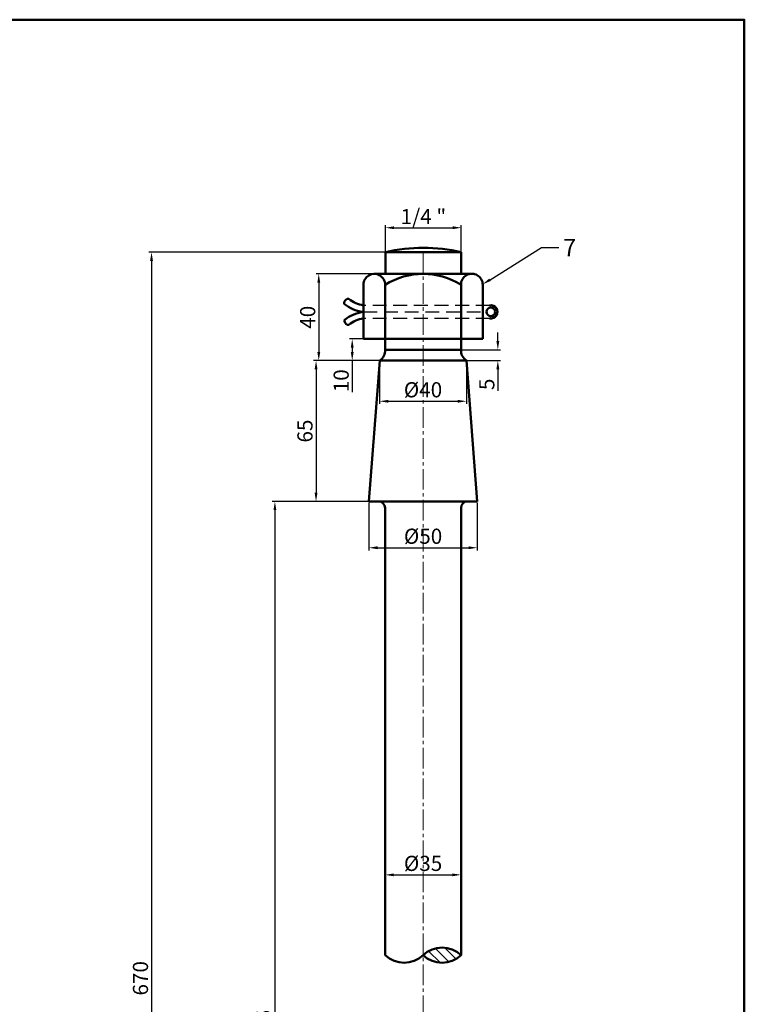
# Model space of a CAD drawing. Units: millimetres. Extents: x -21 to 693, y -570 to 295.
# Tile 7 of 7: x 359 to 693, y -159 to 295. Entities that reach past the tile are written whole.
import ezdxf
from ezdxf import colors
from ezdxf.entities.mleader import LeaderData, LeaderLine
from ezdxf.math import Vec2, Vec3

# ---------------------------------------------------------------- set-up
doc = ezdxf.new("R2010")
doc.units = ezdxf.units.MM
doc.header["$LTSCALE"] = 0.5
doc.linetypes.add('CENTER2', pattern=[28.575, 19.05, -3.175, 3.175, -3.175])
doc.linetypes.add('DASHED', pattern=[19.05, 12.7, -6.35])
for name, color, linetype, lineweight in [('M-CNTR', 1, 'CENTER2', 18), ('M-DIMS', 2, 'Continuous', 25), ('M-HATC', 8, 'Continuous', 18), ('M-HIDN', 6, 'DASHED', 25), ('M-OUTL', 7, 'Continuous', 50), ('M-TEXT', 3, 'Continuous', 25), ('M-TTLB', 7, 'Continuous', 50)]:
    doc.layers.add(name, color=color, linetype=linetype, lineweight=lineweight)
doc.styles.get("Standard").update_dxf_attribs({"font": 'arial.ttf'})
doc.dimstyles.new('ISO-25', dxfattribs={"dimtxt": 7, "dimasz": 4, "dimexe": 1.25, "dimexo": 0.625, "dimtad": 1, "dimdec": 0, "dimtxsty": 'Standard', "dimcen": 2.5, "dimadec": 0, "dimazin": 0, "dimtfac": 1, "dimtdec": 0, "dimtofl": 0, "dimtmove": 0, "dimatfit": 3, "dimfxl": 1, "dimarcsym": 0})

# ---------------------------------------------------------------- blocks, each defined once
blk = doc.blocks.new('*D21')
at = {"layer": 'Defpoints', "color": 0, "ltscale": 0.5, "transparency": 16777216}
for p in [(562.55, 199.43), (527.55, 183.11), (562.55, 183.11)]:
    blk.add_point(p, dxfattribs=at)
at = {"layer": 'M-DIMS', "color": 0, "lineweight": -2, "ltscale": 0.5, "transparency": 16777216}
for p, q in [((527.55, 183.74), (527.55, 200.68)), ((562.55, 183.74), (562.55, 200.68)), ((531.55, 199.43), (558.55, 199.43))]:
    blk.add_line(p, q, dxfattribs=at)
at = {"layer": 'M-DIMS', "color": 0, "ltscale": 0.5, "transparency": 16777216}
for points in [[(531.55, 200.09), (531.55, 198.76), (527.55, 199.43)], [(558.55, 200.09), (558.55, 198.76), (562.55, 199.43)]]:
    blk.add_solid(points, dxfattribs=at)
at = {"layer": 'M-DIMS', "color": 0, "ltscale": 0.5, "transparency": 16777216, "insert": (545.05, 203.67), "char_height": 7, "attachment_point": 5}
blk.add_mtext('1/4 "', dxfattribs=at)
blk = doc.blocks.new('*D22')
at = {"layer": 'Defpoints', "color": 0, "ltscale": 0.5, "transparency": 16777216}
for p in [(530.51, 178.11), (496.77, 138.11), (529.53, 138.11)]:
    blk.add_point(p, dxfattribs=at)
at = {"layer": 'M-DIMS', "color": 0, "lineweight": -2, "ltscale": 0.5, "transparency": 16777216}
for p, q in [((529.88, 178.11), (495.52, 178.11)), ((496.77, 174.11), (496.77, 142.11)), ((528.91, 138.11), (495.52, 138.11))]:
    blk.add_line(p, q, dxfattribs=at)
at = {"layer": 'M-DIMS', "color": 0, "ltscale": 0.5, "transparency": 16777216}
for points in [[(496.11, 174.11), (497.44, 174.11), (496.77, 178.11)], [(496.11, 142.11), (497.44, 142.11), (496.77, 138.11)]]:
    blk.add_solid(points, dxfattribs=at)
at = {"layer": 'M-DIMS', "color": 0, "ltscale": 0.5, "transparency": 16777216, "insert": (492.57, 158.11), "char_height": 7, "attachment_point": 5, "rotation": 90}
blk.add_mtext('40', dxfattribs=at)
blk = doc.blocks.new('*D23')
at = {"layer": 'Defpoints', "color": 0, "ltscale": 0.5, "transparency": 16777216}
for p in [(544.9, 143.11), (544.9, 138.11), (579.4, 138.11)]:
    blk.add_point(p, dxfattribs=at)
at = {"layer": 'M-DIMS', "color": 0, "lineweight": -2, "ltscale": 0.5, "transparency": 16777216}
for p, q in [((579.4, 147.11), (579.4, 151.11)), ((545.53, 143.11), (580.65, 143.11)), ((545.53, 138.11), (580.65, 138.11)), ((579.4, 134.11), (579.4, 124.22))]:
    blk.add_line(p, q, dxfattribs=at)
at = {"layer": 'M-DIMS', "color": 0, "ltscale": 0.5, "transparency": 16777216}
for points in [[(578.73, 147.11), (580.06, 147.11), (579.4, 143.11)], [(578.73, 134.11), (580.06, 134.11), (579.4, 138.11)]]:
    blk.add_solid(points, dxfattribs=at)
at = {"layer": 'M-DIMS', "color": 0, "ltscale": 0.5, "transparency": 16777216, "insert": (575.21, 127.17), "char_height": 7, "attachment_point": 5, "rotation": 90}
blk.add_mtext('5', dxfattribs=at)
blk = doc.blocks.new('*D24')
at = {"layer": 'Defpoints', "color": 0, "ltscale": 0.5, "transparency": 16777216}
for p in [(527.4, 148.11), (512.22, 138.11), (529.53, 138.11)]:
    blk.add_point(p, dxfattribs=at)
at = {"layer": 'M-DIMS', "color": 0, "lineweight": -2, "ltscale": 0.5, "transparency": 16777216}
for p, q in [((526.78, 148.11), (510.97, 148.11)), ((512.22, 144.11), (512.22, 142.11)), ((528.91, 138.11), (510.97, 138.11)), ((512.22, 138.11), (512.22, 123.52))]:
    blk.add_line(p, q, dxfattribs=at)
at = {"layer": 'M-DIMS', "color": 0, "ltscale": 0.5, "transparency": 16777216}
for points in [[(511.55, 144.11), (512.88, 144.11), (512.22, 148.11)], [(511.55, 142.11), (512.88, 142.11), (512.22, 138.11)]]:
    blk.add_solid(points, dxfattribs=at)
at = {"layer": 'M-DIMS', "color": 0, "ltscale": 0.5, "transparency": 16777216, "insert": (508.02, 128.82), "char_height": 7, "attachment_point": 5, "rotation": 90}
blk.add_mtext('10', dxfattribs=at)
blk = doc.blocks.new('*D25')
at = {"layer": 'Defpoints', "color": 0, "ltscale": 0.5, "transparency": 16777216}
for p in [(524.83, 137.14), (564.9, 138.11), (564.9, 119.36)]:
    blk.add_point(p, dxfattribs=at)
at = {"layer": 'M-DIMS', "color": 0, "lineweight": -2, "ltscale": 0.5, "transparency": 16777216}
for p, q in [((524.83, 136.52), (524.83, 118.11)), ((564.9, 137.49), (564.9, 118.11)), ((528.83, 119.36), (560.9, 119.36))]:
    blk.add_line(p, q, dxfattribs=at)
at = {"layer": 'M-DIMS', "color": 0, "ltscale": 0.5, "transparency": 16777216}
for points in [[(528.83, 120.02), (528.83, 118.69), (524.83, 119.36)], [(560.9, 120.02), (560.9, 118.69), (564.9, 119.36)]]:
    blk.add_solid(points, dxfattribs=at)
at = {"layer": 'M-DIMS', "color": 0, "ltscale": 0.5, "transparency": 16777216, "insert": (544.87, 123.75), "char_height": 7, "attachment_point": 5}
blk.add_mtext('%%C40', dxfattribs=at)
blk = doc.blocks.new('*D26')
at = {"layer": 'Defpoints', "color": 0, "ltscale": 0.5, "transparency": 16777216}
for p in [(529.53, 138.11), (495.52, 73.11), (529.53, 73.11)]:
    blk.add_point(p, dxfattribs=at)
at = {"layer": 'M-DIMS', "color": 0, "lineweight": -2, "ltscale": 0.5, "transparency": 16777216}
for p, q in [((528.91, 138.11), (494.27, 138.11)), ((495.52, 134.11), (495.52, 77.11)), ((528.91, 73.11), (494.27, 73.11))]:
    blk.add_line(p, q, dxfattribs=at)
at = {"layer": 'M-DIMS', "color": 0, "ltscale": 0.5, "transparency": 16777216}
for points in [[(494.86, 134.11), (496.19, 134.11), (495.52, 138.11)], [(494.86, 77.11), (496.19, 77.11), (495.52, 73.11)]]:
    blk.add_solid(points, dxfattribs=at)
at = {"layer": 'M-DIMS', "color": 0, "ltscale": 0.5, "transparency": 16777216, "insert": (491.32, 105.61), "char_height": 7, "attachment_point": 5, "rotation": 90}
blk.add_mtext('65', dxfattribs=at)
blk = doc.blocks.new('*D27')
at = {"layer": 'Defpoints', "color": 0, "ltscale": 0.5, "transparency": 16777216}
for p in [(519.9, 73.11), (569.9, 73.11), (569.9, 51.77)]:
    blk.add_point(p, dxfattribs=at)
at = {"layer": 'M-DIMS', "color": 0, "lineweight": -2, "ltscale": 0.5, "transparency": 16777216}
for p, q in [((519.9, 72.49), (519.9, 50.52)), ((569.9, 72.49), (569.9, 50.52)), ((523.9, 51.77), (565.9, 51.77))]:
    blk.add_line(p, q, dxfattribs=at)
at = {"layer": 'M-DIMS', "color": 0, "ltscale": 0.5, "transparency": 16777216}
for points in [[(523.9, 52.44), (523.9, 51.11), (519.9, 51.77)], [(565.9, 52.44), (565.9, 51.11), (569.9, 51.77)]]:
    blk.add_solid(points, dxfattribs=at)
at = {"layer": 'M-DIMS', "color": 0, "ltscale": 0.5, "transparency": 16777216, "insert": (544.9, 56.17), "char_height": 7, "attachment_point": 5}
blk.add_mtext('%%C50', dxfattribs=at)
blk = doc.blocks.new('*D28')
at = {"layer": 'Defpoints', "color": 0, "ltscale": 0.5, "transparency": 16777216}
for p in [(545.05, 188.11), (419.62, -481.89), (545.05, -481.89)]:
    blk.add_point(p, dxfattribs=at)
at = {"layer": 'M-DIMS', "color": 0, "lineweight": -2, "ltscale": 0.5, "transparency": 16777216}
for p, q in [((544.43, 188.11), (418.37, 188.11)), ((419.62, 184.11), (419.62, -477.89)), ((544.43, -481.89), (418.37, -481.89))]:
    blk.add_line(p, q, dxfattribs=at)
at = {"layer": 'M-DIMS', "color": 0, "ltscale": 0.5, "transparency": 16777216}
for points in [[(418.95, 184.11), (420.29, 184.11), (419.62, 188.11)], [(418.95, -477.89), (420.29, -477.89), (419.62, -481.89)]]:
    blk.add_solid(points, dxfattribs=at)
at = {"layer": 'M-DIMS', "color": 0, "ltscale": 0.5, "transparency": 16777216, "insert": (415.42, -146.89), "char_height": 7, "attachment_point": 5, "rotation": 90}
blk.add_mtext('670', dxfattribs=at)
blk = doc.blocks.new('*D29')
at = {"layer": 'Defpoints', "color": 0, "ltscale": 0.5, "transparency": 16777216}
for p in [(511.59, 73.11), (476.54, -411.89), (528.15, -411.89)]:
    blk.add_point(p, dxfattribs=at)
at = {"layer": 'M-DIMS', "color": 0, "lineweight": -2, "ltscale": 0.5, "transparency": 16777216}
for p, q in [((510.97, 73.11), (475.29, 73.11)), ((476.54, 69.11), (476.54, -407.89)), ((527.53, -411.89), (475.29, -411.89))]:
    blk.add_line(p, q, dxfattribs=at)
at = {"layer": 'M-DIMS', "color": 0, "ltscale": 0.5, "transparency": 16777216}
for points in [[(475.87, 69.11), (477.21, 69.11), (476.54, 73.11)], [(475.87, -407.89), (477.21, -407.89), (476.54, -411.89)]]:
    blk.add_solid(points, dxfattribs=at)
at = {"layer": 'M-DIMS', "color": 0, "ltscale": 0.5, "transparency": 16777216, "insert": (472.34, -169.39), "char_height": 7, "attachment_point": 5, "rotation": 90}
blk.add_mtext('485', dxfattribs=at)
blk = doc.blocks.new('*D30')
at = {"layer": 'Defpoints', "color": 0, "ltscale": 0.5, "transparency": 16777216}
for p in [(527.4, -98.55), (562.4, -98.55), (562.4, -99.16)]:
    blk.add_point(p, dxfattribs=at)
at = {"layer": 'M-DIMS', "color": 0, "lineweight": -2, "ltscale": 0.5, "transparency": 16777216}
for p, q in [((527.4, -99.18), (527.4, -100.41)), ((531.4, -99.16), (558.4, -99.16)), ((562.4, -99.18), (562.4, -100.41))]:
    blk.add_line(p, q, dxfattribs=at)
at = {"layer": 'M-DIMS', "color": 0, "ltscale": 0.5, "transparency": 16777216}
for points in [[(531.4, -98.5), (531.4, -99.83), (527.4, -99.16)], [(558.4, -98.5), (558.4, -99.83), (562.4, -99.16)]]:
    blk.add_solid(points, dxfattribs=at)
at = {"layer": 'M-DIMS', "color": 0, "ltscale": 0.5, "transparency": 16777216, "insert": (544.9, -94.77), "char_height": 7, "attachment_point": 5}
blk.add_mtext('%%C35', dxfattribs=at)

msp = doc.modelspace()

# ---------------------------------------------------------------- hatches: boundary and pattern name
at = {"layer": 'M-HATC', "ltscale": 0.5}
h = msp.add_hatch(dxfattribs=at)
h.set_pattern_fill('ANSI31', color=256, angle=90)
h.paths.add_polyline_path([(562.403, -136.2127, 0.39671485), (544.903, -136.2127, 0.39671485)])
h.paths.add_polyline_path([(544.903, -170.8866, -0.39671485), (527.403, -170.8866, -0.39671485)])
h.paths.add_polyline_path([(544.903, -464.8866), (528.903, -464.8866), (528.903, -481.8866), (544.903, -481.8866)])
h.paths.add_polyline_path([(560.903, -464.8866), (544.903, -464.8866), (544.903, -481.8866), (560.903, -481.8866)])

# ---------------------------------------------------------------- linework, layer by layer
at = {"layer": 'M-CNTR'}
msp.add_line((544.903, 188.1134), (544.903, -481.8866), dxfattribs=at)
at = {"layer": 'M-HIDN'}
for p, q in [((575.6231, 163.6183), (517.403, 163.6183)), ((517.403, 160.6183), (574.1551, 160.6183)), ((575.6231, 157.6183), (517.403, 157.6183))]:
    msp.add_line(p, q, dxfattribs=at)
at = {"layer": 'M-OUTL'}
for p, q in [((527.5534, 178.1134), (527.5534, 188.1134)), ((527.5534, 188.1134), (562.5534, 188.1134)), ((562.5534, 188.1134), (562.5534, 178.1134)), ((568.4203, 178.1134), (522.1811, 178.1134)), ((517.403, 173.1232), (517.403, 148.1134)), ((527.403, 173.1232), (527.403, 148.1134)), ((562.403, 148.1134), (562.403, 173.3203)), ((572.403, 148.1134), (572.403, 173.3203)), ((517.403, 148.1134), (572.403, 148.1134)), ((527.403, 148.1134), (527.403, 143.1134)), ((562.403, 143.1134), (562.403, 148.1134)), ((527.403, 143.1134), (562.403, 143.1134)), ((524.903, 138.1134), (519.903, 73.1134)), ((524.903, 138.1134), (564.903, 138.1134)), ((564.903, 138.1134), (569.903, 73.1134)), ((519.903, 73.1134), (569.903, 73.1134)), ((527.403, -136.2127), (527.403, 70.1134)), ((562.403, -136.2127), (562.403, 70.1134))]:
    msp.add_line(p, q, dxfattribs=at)
msp.add_circle((576.1922, 160.6183), 2.0371, dxfattribs=at)
for centre, radius, start, end in [((545.0534, 115.5045), 74.688, 76.449165, 103.550835), ((522.403, 173.1183), 5, 359.943578, 180.056422), ((544.8951, 144.9606), 33.1527, 58.1229, 121.844859), ((567.403, 173.2169), 5.0011, 358.814236, 181.185764), ((576.1922, 160.6183), 3.0535, 259.258021, 100.741979), ((521.8832, 142.7483), 5.5319, 303.085741, 3.784156), ((567.9229, 142.7483), 5.5319, 176.215844, 236.914259), ((524.403, 70.1134), 3, 0, 90), ((565.403, 70.1134), 3, 90, 180), ((536.153, -126.9203), 12.7637, 226.722074, 313.277926), ((553.653, -145.5052), 12.7637, 46.722074, 133.277926), ((553.653, -126.9203), 12.7637, 226.722074, 313.277926)]:
    msp.add_arc(centre, radius, start, end, dxfattribs=at)
at = {"layer": 'M-OUTL', "ltscale": 0.5}
for centre, radius, start, end in [((519.5243, 177.7803), 17.4171, 231.413176, 261.481097), ((519.5243, 177.7803), 14.32, 231.413176, 261.481097), ((519.5243, 143.4563), 17.2869, 98.518903, 128.586824), ((519.5243, 143.4563), 14.32, 98.518903, 128.586824)]:
    msp.add_arc(centre, radius, start, end, dxfattribs=at)
at = {"layer": 'M-OUTL'}
for points in [[(508.6613, 164.166), (507.8543, 164.8099), (509.786, 167.2308), (510.593, 166.5869)], [(508.7425, 156.9688), (507.9695, 156.352), (509.8199, 154.0329), (510.593, 154.6497)]]:
    msp.add_open_spline(points, degree=3, dxfattribs=at)
at = {"layer": 'M-TTLB', "ltscale": 0.5}
msp.add_lwpolyline([(-21.49, 295.4176), (693.1139, 295.4176), (693.1139, -570.0874), (-21.49, -570.0874)], close=True, dxfattribs=at)

# ---------------------------------------------------------------- dimensions: what is measured, and where the dimension line sits
at = {"layer": 'M-DIMS', "ltscale": 0.5}
for base, p1, p2, text, picture, middle in [((562.5534, 199.4266), (527.5534, 183.1134), (562.5534, 183.1134), '1/4 "', '*D21', (545.0534, 203.671)), ((564.903, 119.3572), (524.8284, 137.1431), (564.903, 138.1134), '%%C<>', '*D25', (544.8657, 123.752)), ((569.903, 51.7743), (519.903, 73.1134), (569.903, 73.1134), '%%C<>', '*D27', (544.903, 56.1691)), ((562.403, -99.1649), (527.403, -98.5512), (562.403, -98.5512), '%%C<>', '*D30', (544.903, -94.7701))]:
    dim = msp.add_linear_dim(base=base, p1=p1, p2=p2, text=text, dimstyle='ISO-25', override={"dimclrd": 0, "dimclre": 0, "dimclrt": 0}, dxfattribs=at)
    dim.commit()
    dim.dimension.update_dxf_attribs({"geometry": picture, "text_midpoint": middle})
for base, p1, p2, picture, middle in [((419.6197, -481.8866), (545.0534, 188.1134), (545.0534, -481.8866), '*D28', (415.4207, -146.8866)), ((496.7726, 138.1134), (530.5064, 178.1134), (529.5331, 138.1134), '*D22', (492.5736, 158.1134)), ((579.3979, 138.1134), (544.903, 143.1134), (544.903, 138.1134), '*D23', (575.2133, 127.1678)), ((512.2153, 138.1134), (527.403, 148.1134), (529.5331, 138.1134), '*D24', (508.0163, 128.8161)), ((495.5226, 73.1134), (529.5331, 138.1134), (529.5331, 73.1134), '*D26', (491.3236, 105.6134)), ((476.5413, -411.8866), (511.5903, 73.1134), (528.153, -411.8866), '*D29', (472.3422, -169.3866))]:
    dim = msp.add_linear_dim(base=base, p1=p1, p2=p2, angle=90, dimstyle='ISO-25', override={"dimclrd": 0, "dimclre": 0, "dimclrt": 0}, dxfattribs=at)
    dim.commit()
    dim.dimension.update_dxf_attribs({"geometry": picture, "text_midpoint": middle})

# ---------------------------------------------------------------- leaders
at = {"layer": 'M-TEXT', "ltscale": 0.5}
ml = msp.add_multileader_mtext('Standard', dxfattribs=at)
ml.set_content('7', color=256)
ml.set_leader_properties()
ml.build(insert=Vec2(0, 0))
ctx = ml.context
ctx.base_point, ctx.char_height, ctx.plane_origin = Vec3(607.4719, 190.2429), 8, Vec3(572.403, 173.3203)
notes = []
notes.append((ctx, [(0, (1, 1, 0), (599.4719, 190.2429), (1, 0), 8, [(0, [(572.403, 173.3203)], 0, [])])]))
ctx.mtext.insert, ctx.mtext.flow_direction = Vec3(609.4719, 194.2429), 5
for ctx, leaders in notes:
    for number, flags, end, landing, length, lines in leaders:
        leader = LeaderData()
        leader.index, (leader.has_last_leader_line, leader.has_dogleg_vector, leader.attachment_direction) = number, flags
        leader.last_leader_point, leader.dogleg_vector, leader.dogleg_length = Vec3(end), Vec3(landing), length
        for number, points, colour, breaks in lines:
            line = LeaderLine()
            line.index, line.vertices, line.color, line.breaks = number, Vec3.list(points), colors.encode_raw_color(colour), breaks
            leader.lines.append(line)
        ctx.leaders.append(leader)

doc.saveas('drawing.dxf')
